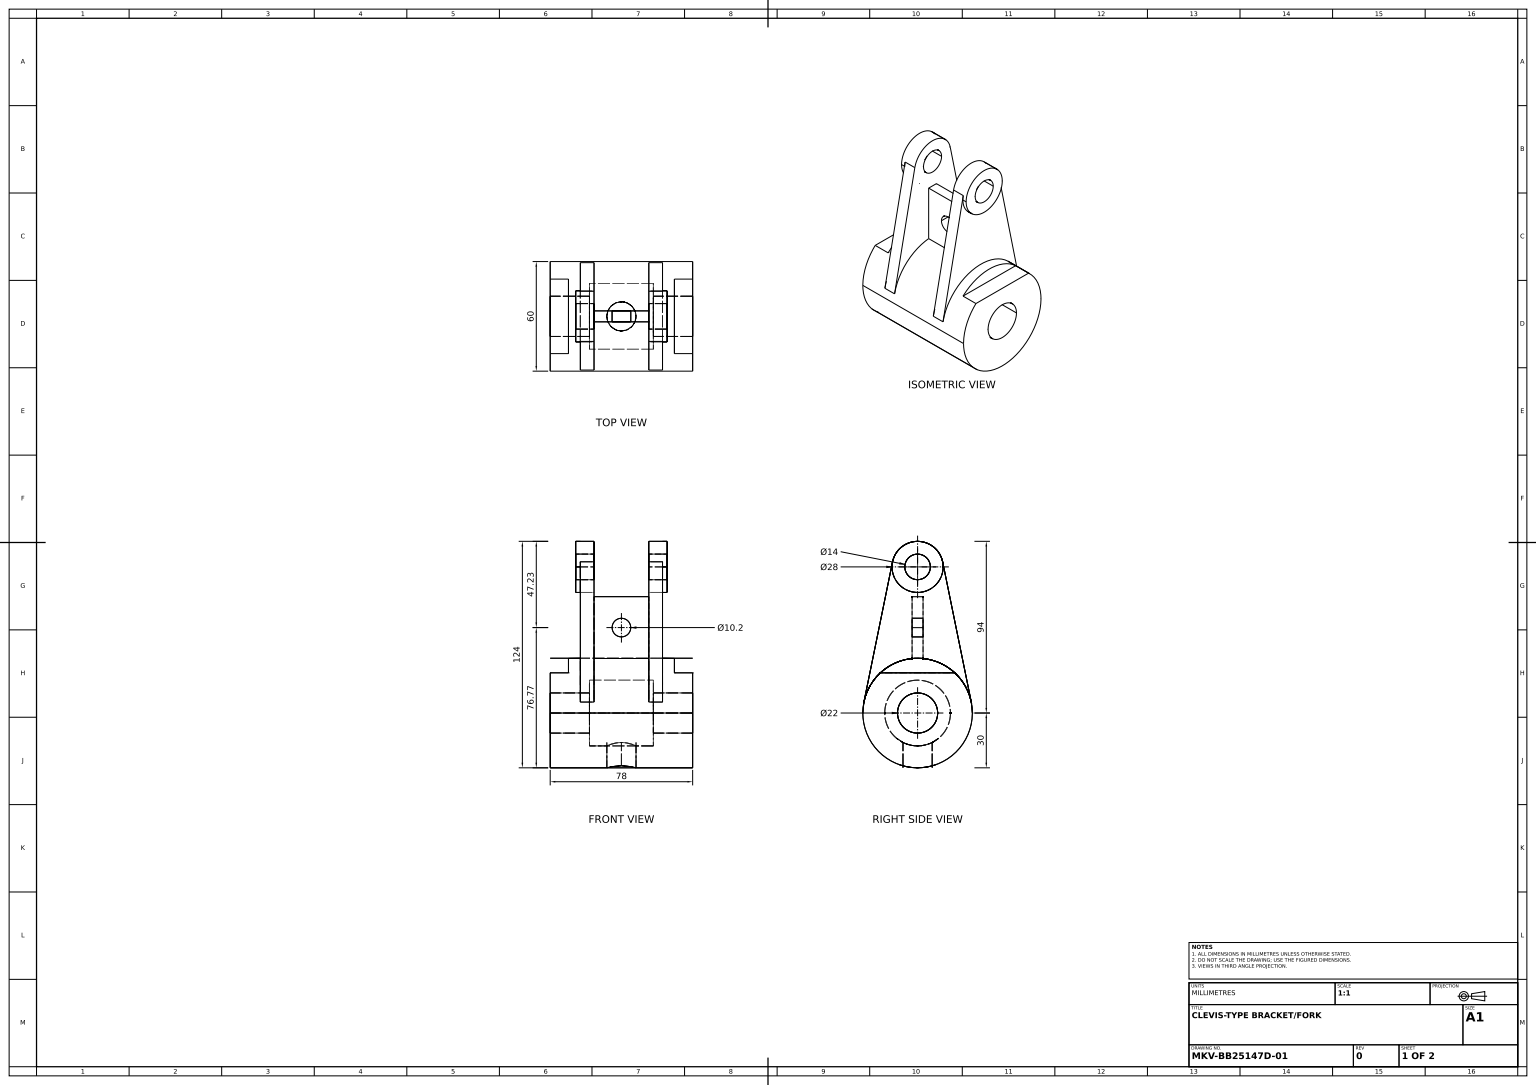
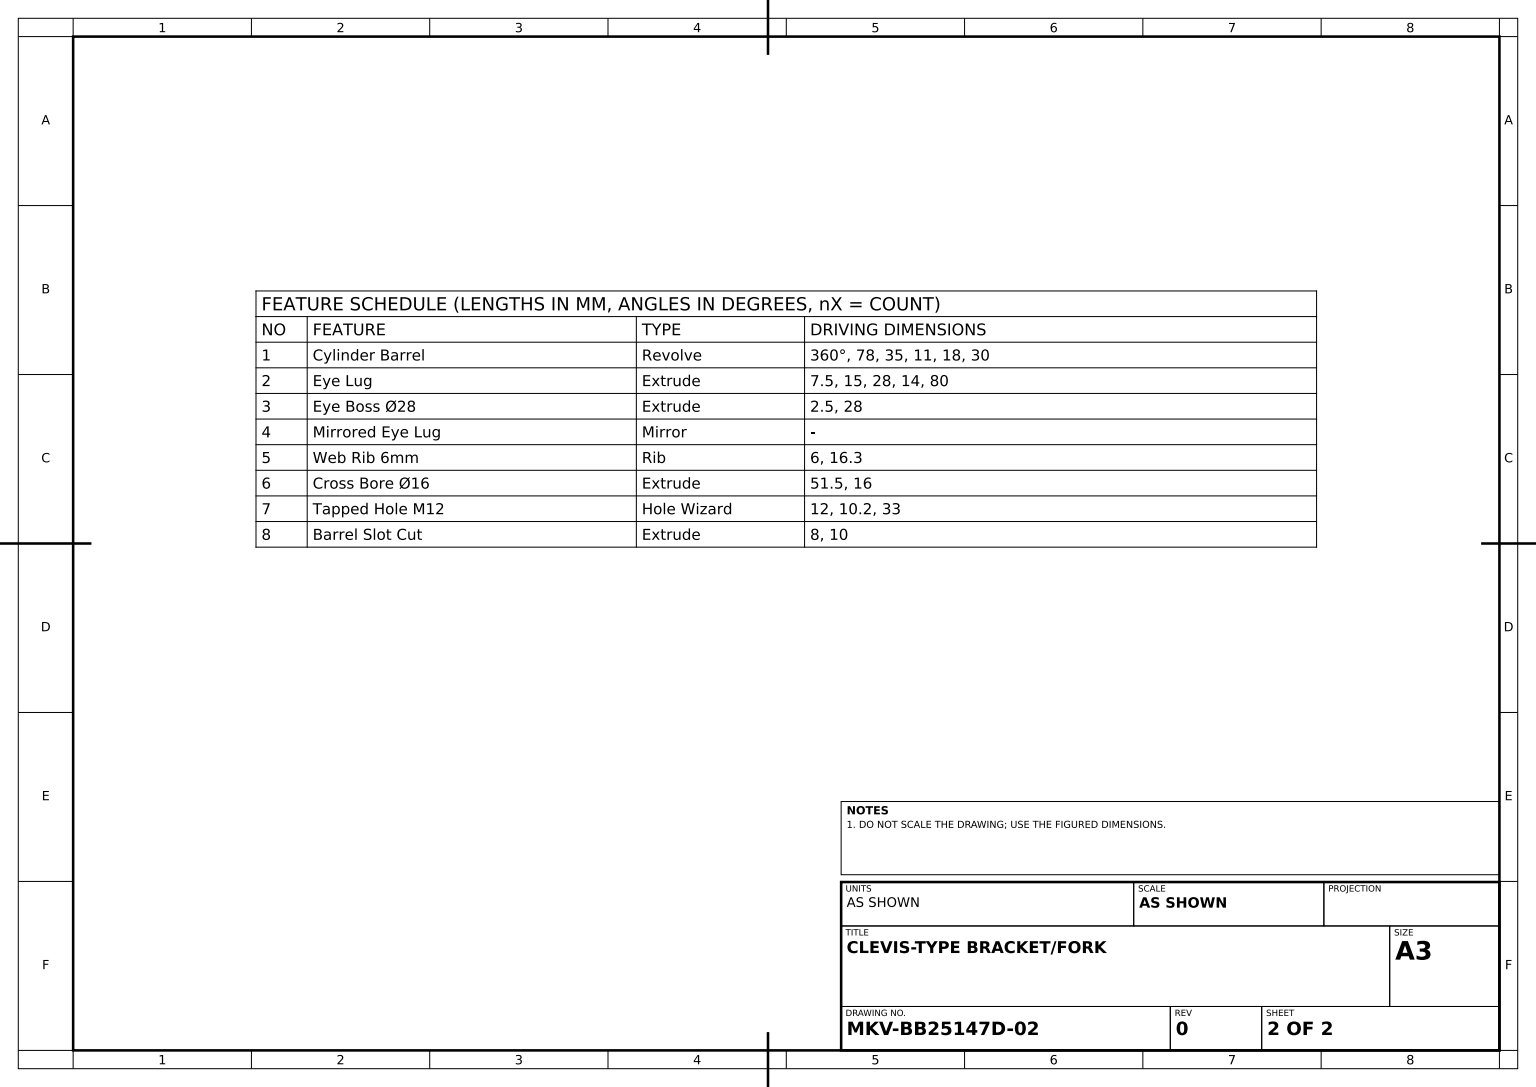
SolidWorks part; units mm, degrees
material "Plain Carbon Steel"
ref_plane "Front Plane" through (0, 0, 0) normal (0, 0, 1) x (1, 0, 0)
ref_plane "Top Plane" through (0, 0, 0) normal (0, 1, 0) x (1, 0, 0)
ref_plane "Right Plane" through (0, 0, 0) normal (1, 0, 0) x (0, 0, -1)
sketch "Barrel Profile Sketch" plane through (0, 0, 0) normal (0, 0, 1) x (1, 0, 0)
  line L0 (-46.634, 0) -> (47.8511, 0) construction
  line L1 (-39, 11) -> (-39, 30)
  line L2 (-39, 30) -> (39, 30)
  line L3 (39, 30) -> (39, 11)
  line L4 (39, 11) -> (17.5, 11)
  line L5 (17.5, 11) -> (17.5, 18)
  line L6 (17.5, 18) -> (-17.5, 18)
  line L7 (-17.5, 18) -> (-17.5, 11)
  line L8 (-17.5, 11) -> (-39, 11)
  line L9 (0, 0) -> (0, 28.3787) construction
  dimension "D1" = 78
  dimension "D2" = 11
  dimension "D3" = 18
  dimension "D4" = 30
  dimension "D5" = 35
revolve "Cylinder Barrel" add sketch "Barrel Profile Sketch" angle 360 about L0
sketch "Eye Lug Sketch" plane through (0, 0, 0) normal (1, 0, 0) x (0, 0, -1)
  line L0 (0, 0) -> (0, 80) construction
  line L1 (-29.3939, 6) -> (-13.7171, 82.8)
  line L2 (29.3939, 6) -> (13.7171, 82.8)
  arc A0 (13.7171, 82.8) -> (-13.7171, 82.8) centre (0, 80) ccw
  circle A1 centre (0, 80) radius 7
  circle A2 centre (0, 0) radius 30 construction
  arc A3 (29.3939, 6) -> (-29.3939, 6) centre (0, 0) ccw
  dimension "D1" = 28
  dimension "D2" = 14
  dimension "D3" = 80
extrude "Eye Lug" add sketch "Eye Lug Sketch" along normal blind 7.5 from offset 15
sketch "Eye Boss Sketch" plane through (22.5, 0, 0) normal (1, 0, 0) x (0, 0, -1)
  circle A0 centre (0, 80) radius 14
  circle A1 centre (0, 80) radius 7 construction
  circle A2 centre (0, 80) radius 7
  dimension "D1" = 28
extrude "Eye Boss Ø28" add sketch "Eye Boss Sketch" along normal blind 2.5
mirror "Mirrored Eye Lug" about plane through (0, 0, 0) normal (1, 0, 0) of "Eye Lug", "Eye Boss Ø28"
sketch "Web Rib Sketch" plane through (0, 0, 0) normal (0, 0, 1) x (1, 0, 0)
  line L0 (-15, 63.7) -> (15, 63.7)
  line L1 (-15, 82.8) -> (-15, 6) construction
  line L2 (15, 82.8) -> (15, 6) construction
  line L3 (-25, 80) -> (25, 80) construction
  line L4 (-25, 94) -> (-25, 66) construction
  line L5 (25, 66) -> (25, 94) construction
  dimension "D1" = 16.3
rib "Web Rib 6mm" sketch "Web Rib Sketch" sketch "Web Rib Sketch" thickness 6 extrusion direction parallel to sketch draft on no parameters "D1"=6
sketch "Cross Bore Sketch" plane through (0, 0, 0) normal (0, 1, 0) x (1, 0, 0)
  circle A0 centre (0, 0) radius 8
  dimension "D1" = 16
extrude "Cross Bore Ø16" cut sketch "Cross Bore Sketch" against normal blind 51.5
hole_wizard "Tapped Hole M12" positions "3DSketch1" profile "Sketch6" tap size "M12" standard "ISO" end condition through all
sketch3d "3DSketch1"
  line L0 (-15, 63.7, 3) -> (15, 63.7, 3) construction
  line L1 (-15, 29.8496, 3) -> (-15, 63.7, 3) construction
  point P0 (0, 46.7748, 3)
  point P5 (0, 63.7, 3)
  point P8 (-15, 46.7748, 3)
sketch "Sketch6" plane through (0, 46.7748, 3) normal (1, 0, 0) x (0, -1, 0)
  line L0 (0, 0) -> (0, 33)
  line L1 (0, 33) -> (5.1, 33)
  line L2 (5.1, 33) -> (5.1, 0)
  line L5 (5.1, 0) -> (0, 0)
  line L11 (0, -6.35) -> (0, 107.95) construction
  dimension "Thru Tap Drill Dia." = 10.2
  dimension "Thru Tap Drill Depth" = 33
cosmetic thread "Hole Thread1" parameters "D2"=12
sketch "Barrel Slot Sketch" plane through (0, 0, 0) normal (0, 0, 1) x (1, 0, 0)
  line L1 (-39, 30) -> (-29, 30)
  line L2 (-39, 30) -> (-39, 22)
  line L3 (-39, 22) -> (-29, 22)
  line L4 (-29, 30) -> (-29, 22)
  line L5 (39, 30) -> (29, 30)
  line L6 (39, 30) -> (39, 22)
  line L7 (39, 22) -> (29, 22)
  line L8 (29, 30) -> (29, 22)
  dimension "D1" = 8
  dimension "D2" = 10
extrude "Barrel Slot Cut" cut sketch "Barrel Slot Sketch" against normal through all both and the other way through all
